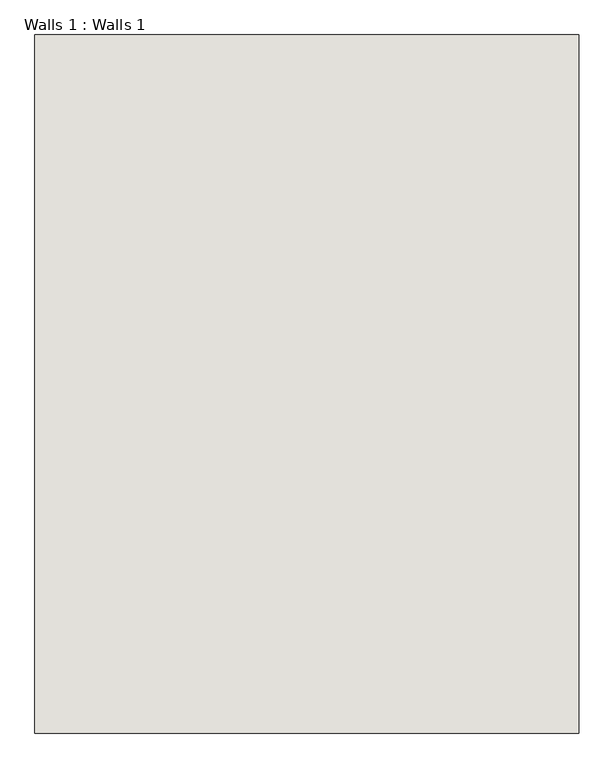
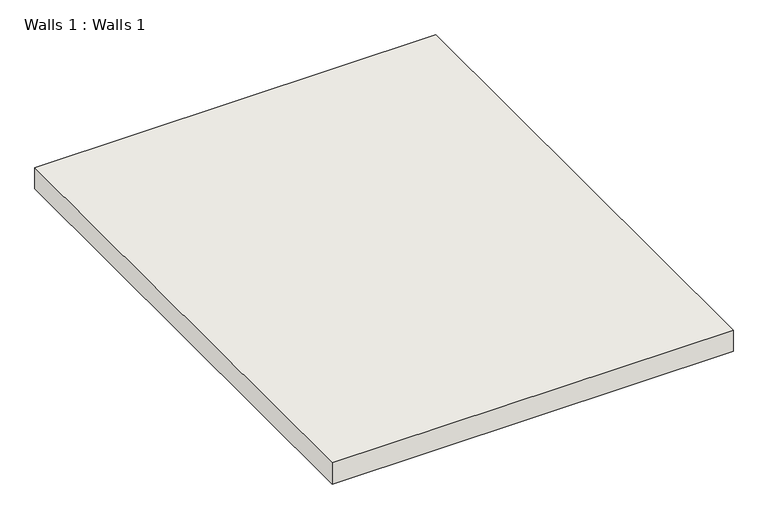
"""IFC4 building model written with IfcOpenShell, lengths in millimetres: wall geometry, Walls 1 : Walls 1."""

from ifc_helpers import new_model, si_unit, frame, origin, place, context, project, spatial, polyline, outline, extrude, source, transform, mapped, element, save


def walls_1_walls_1_3090deb3(model_context):
    return source(origin(), model_context, "Body", "SweptSolid", [
        extrude(outline(polyline([(-6951.0772223, -5400.2511748), (-6951.0772223, -20223.5461067), (-18499.7074219, -20223.5461067), (-18499.7074219, -5400.2511748), (-6951.0772223, -5400.2511748)])), frame((0.0, 0.0, 5648.0), z_axis=(0.0, 0.0, 1.0), x_axis=(1.0, 0.0, 0.0)), (0.0, 0.0, 1.0), 643.756289),
    ])


if __name__ == "__main__":
    model = new_model("IFC4")
    model_context = context("Model", 3, world=origin())
    ifc_project = project(units=[si_unit("LENGTHUNIT", "METRE", prefix="MILLI")], contexts=[model_context])
    site = spatial("IfcSite", under=ifc_project)
    building = spatial("IfcBuilding", under=site)
    placement = place(None, origin())
    walls_1_walls_1_shape = walls_1_walls_1_3090deb3(model_context)
    element("IfcWall", 1, ObjectType="Walls 1 : Walls 1", at=placement, inside=building, context=model_context, shape_type="MappedRepresentation", body=[
        mapped(walls_1_walls_1_shape, transform((0.0, 0.0, 0.0), x_axis=(1.0, 0.0, 0.0), y_axis=(0.0, 1.0, 0.0), z_axis=(0.0, 0.0, 1.0))),
    ])
    save(model, "model.ifc")

# Revit data of these elements
# Element 1 (IfcWall, "Walls 1 : Walls 1")
#   Materials on its faces: "Default Wall"
# Materials
#   "Default Wall": colour RGB 80 80 80, transparency 0
